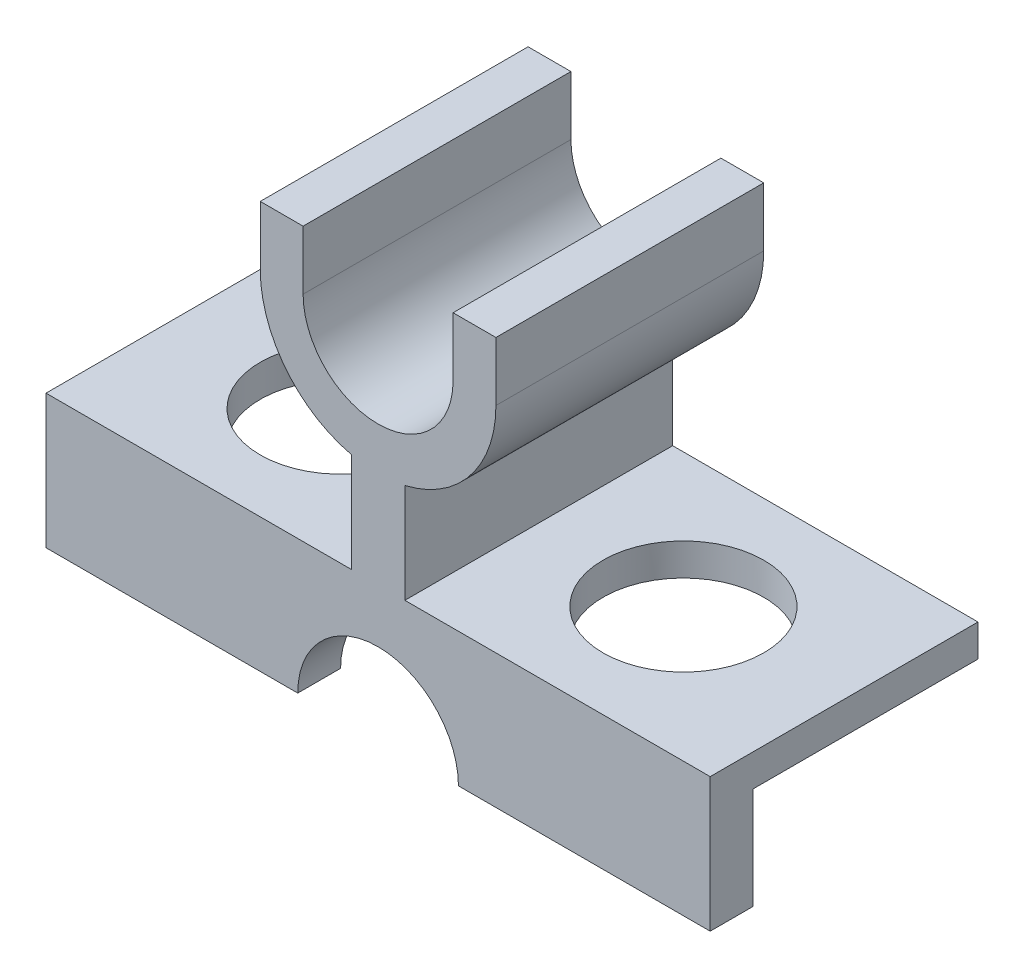
ISO-10303-21;
HEADER;
FILE_DESCRIPTION(('STEP AP214'),'2;1');
FILE_NAME('part.step','',(''),(''),'','','');
FILE_SCHEMA(('AUTOMOTIVE_DESIGN { 1 0 10303 214 1 1 1 1 }'));
ENDSEC;
DATA;
#1=APPLICATION_CONTEXT('core data for automotive mechanical design processes');
#2=APPLICATION_PROTOCOL_DEFINITION('international standard','automotive_design',2000,#1);
#3=PRODUCT_CONTEXT('',#1,'mechanical');
#4=PRODUCT('Part','Part','',(#3));
#5=PRODUCT_RELATED_PRODUCT_CATEGORY('part','',(#4));
#6=PRODUCT_DEFINITION_FORMATION('','',#4);
#7=PRODUCT_DEFINITION_CONTEXT('part definition',#1,'design');
#8=PRODUCT_DEFINITION('design','',#6,#7);
#9=PRODUCT_DEFINITION_SHAPE('','',#8);
#10=(LENGTH_UNIT() NAMED_UNIT(*) SI_UNIT(.MILLI.,.METRE.));
#11=(NAMED_UNIT(*) PLANE_ANGLE_UNIT() SI_UNIT($,.RADIAN.));
#12=(NAMED_UNIT(*) SI_UNIT($,.STERADIAN.) SOLID_ANGLE_UNIT());
#13=UNCERTAINTY_MEASURE_WITH_UNIT(LENGTH_MEASURE(1.E-05),#10,'distance_accuracy_value','');
#14=(GEOMETRIC_REPRESENTATION_CONTEXT(3) GLOBAL_UNCERTAINTY_ASSIGNED_CONTEXT((#13)) GLOBAL_UNIT_ASSIGNED_CONTEXT((#10,
#11,#12)) REPRESENTATION_CONTEXT('',''));
#15=CARTESIAN_POINT('',(0.,0.,0.));
#16=DIRECTION('',(0.,0.,1.));
#17=DIRECTION('',(1.,0.,0.));
#18=AXIS2_PLACEMENT_3D('',#15,#16,#17);
#19=CARTESIAN_POINT('',(-62.,0.,25.));
#20=DIRECTION('',(1.,0.,0.));
#21=DIRECTION('',(0.,0.,-1.));
#22=AXIS2_PLACEMENT_3D('',#19,#20,#21);
#23=PLANE('',#22);
#24=DIRECTION('',(0.,0.,1.));
#25=VECTOR('',#24,1.);
#26=CARTESIAN_POINT('',(-62.,19.,-25.));
#27=LINE('',#26,#25);
#28=CARTESIAN_POINT('',(-62.,19.,-25.));
#29=VERTEX_POINT('',#28);
#30=CARTESIAN_POINT('',(-62.,19.,17.));
#31=VERTEX_POINT('',#30);
#32=EDGE_CURVE('E54',#29,#31,#27,.T.);
#33=ORIENTED_EDGE('',*,*,#32,.T.);
#34=DIRECTION('',(0.,-1.,0.));
#35=VECTOR('',#34,1.);
#36=CARTESIAN_POINT('',(-62.,0.,17.));
#37=LINE('',#36,#35);
#38=CARTESIAN_POINT('',(-62.,0.,17.));
#39=VERTEX_POINT('',#38);
#40=EDGE_CURVE('E284',#31,#39,#37,.T.);
#41=ORIENTED_EDGE('',*,*,#40,.T.);
#42=DIRECTION('',(0.,0.,-1.));
#43=VECTOR('',#42,1.);
#44=CARTESIAN_POINT('',(-62.,0.,25.));
#45=LINE('',#44,#43);
#46=CARTESIAN_POINT('',(-62.,0.,25.));
#47=VERTEX_POINT('',#46);
#48=EDGE_CURVE('E50',#47,#39,#45,.T.);
#49=ORIENTED_EDGE('',*,*,#48,.F.);
#50=DIRECTION('',(0.,-1.,0.));
#51=VECTOR('',#50,1.);
#52=CARTESIAN_POINT('',(-62.,0.,25.));
#53=LINE('',#52,#51);
#54=CARTESIAN_POINT('',(-62.,25.,25.));
#55=VERTEX_POINT('',#54);
#56=EDGE_CURVE('E230',#55,#47,#53,.T.);
#57=ORIENTED_EDGE('',*,*,#56,.F.);
#58=DIRECTION('',(0.,0.,-1.));
#59=VECTOR('',#58,1.);
#60=CARTESIAN_POINT('',(-62.,25.,25.));
#61=LINE('',#60,#59);
#62=CARTESIAN_POINT('',(-62.,25.,-25.));
#63=VERTEX_POINT('',#62);
#64=EDGE_CURVE('E195',#55,#63,#61,.T.);
#65=ORIENTED_EDGE('',*,*,#64,.T.);
#66=DIRECTION('',(0.,-1.,0.));
#67=VECTOR('',#66,1.);
#68=CARTESIAN_POINT('',(-62.,0.,-25.));
#69=LINE('',#68,#67);
#70=EDGE_CURVE('E197',#63,#29,#69,.T.);
#71=ORIENTED_EDGE('',*,*,#70,.T.);
#72=EDGE_LOOP('',(#33,#41,#49,#57,#65,#71));
#73=FACE_BOUND('',#72,.T.);
#74=ADVANCED_FACE('F39',(#73),#23,.F.);
#75=CARTESIAN_POINT('',(-62.,0.,25.));
#76=DIRECTION('',(0.,1.,0.));
#77=DIRECTION('',(0.,0.,1.));
#78=AXIS2_PLACEMENT_3D('',#75,#76,#77);
#79=PLANE('',#78);
#80=ORIENTED_EDGE('',*,*,#48,.T.);
#81=DIRECTION('',(1.,0.,0.));
#82=VECTOR('',#81,1.);
#83=CARTESIAN_POINT('',(-62.,0.,17.));
#84=LINE('',#83,#82);
#85=CARTESIAN_POINT('',(-15.,0.,17.));
#86=VERTEX_POINT('',#85);
#87=EDGE_CURVE('E286',#39,#86,#84,.T.);
#88=ORIENTED_EDGE('',*,*,#87,.T.);
#89=DIRECTION('',(0.,0.,-1.));
#90=VECTOR('',#89,1.);
#91=CARTESIAN_POINT('',(-15.,0.,25.));
#92=LINE('',#91,#90);
#93=CARTESIAN_POINT('',(-15.,0.,25.));
#94=VERTEX_POINT('',#93);
#95=EDGE_CURVE('E270',#94,#86,#92,.T.);
#96=ORIENTED_EDGE('',*,*,#95,.F.);
#97=DIRECTION('',(1.,0.,0.));
#98=VECTOR('',#97,1.);
#99=CARTESIAN_POINT('',(-62.,0.,25.));
#100=LINE('',#99,#98);
#101=EDGE_CURVE('E121',#47,#94,#100,.T.);
#102=ORIENTED_EDGE('',*,*,#101,.F.);
#103=EDGE_LOOP('',(#80,#88,#96,#102));
#104=FACE_BOUND('',#103,.T.);
#105=ADVANCED_FACE('F350',(#104),#79,.F.);
#106=CARTESIAN_POINT('',(0.,0.,25.));
#107=DIRECTION('',(0.,0.,-1.));
#108=DIRECTION('',(-1.,0.,0.));
#109=AXIS2_PLACEMENT_3D('',#106,#107,#108);
#110=CYLINDRICAL_SURFACE('',#109,15.);
#111=ORIENTED_EDGE('',*,*,#95,.T.);
#112=CARTESIAN_POINT('',(0.,0.,17.));
#113=DIRECTION('',(0.,0.,1.));
#114=DIRECTION('',(1.,0.,0.));
#115=AXIS2_PLACEMENT_3D('',#112,#113,#114);
#116=CIRCLE('',#115,15.);
#117=CARTESIAN_POINT('',(15.,0.,17.));
#118=VERTEX_POINT('',#117);
#119=EDGE_CURVE('E203',#86,#118,#116,.F.);
#120=ORIENTED_EDGE('',*,*,#119,.T.);
#121=DIRECTION('',(0.,0.,-1.));
#122=VECTOR('',#121,1.);
#123=CARTESIAN_POINT('',(15.,0.,25.));
#124=LINE('',#123,#122);
#125=CARTESIAN_POINT('',(15.,0.,25.));
#126=VERTEX_POINT('',#125);
#127=EDGE_CURVE('E262',#126,#118,#124,.T.);
#128=ORIENTED_EDGE('',*,*,#127,.F.);
#129=CARTESIAN_POINT('',(0.,0.,25.));
#130=DIRECTION('',(0.,0.,-1.));
#131=DIRECTION('',(-1.,0.,0.));
#132=AXIS2_PLACEMENT_3D('',#129,#130,#131);
#133=CIRCLE('',#132,15.);
#134=EDGE_CURVE('E301',#94,#126,#133,.T.);
#135=ORIENTED_EDGE('',*,*,#134,.F.);
#136=EDGE_LOOP('',(#111,#120,#128,#135));
#137=FACE_BOUND('',#136,.T.);
#138=ADVANCED_FACE('F351',(#137),#110,.F.);
#139=CARTESIAN_POINT('',(15.,0.,25.));
#140=DIRECTION('',(0.,1.,0.));
#141=DIRECTION('',(0.,0.,1.));
#142=AXIS2_PLACEMENT_3D('',#139,#140,#141);
#143=PLANE('',#142);
#144=ORIENTED_EDGE('',*,*,#127,.T.);
#145=CARTESIAN_POINT('',(62.,0.,17.));
#146=VERTEX_POINT('',#145);
#147=EDGE_CURVE('E291',#118,#146,#84,.T.);
#148=ORIENTED_EDGE('',*,*,#147,.T.);
#149=DIRECTION('',(0.,0.,-1.));
#150=VECTOR('',#149,1.);
#151=CARTESIAN_POINT('',(62.,0.,25.));
#152=LINE('',#151,#150);
#153=CARTESIAN_POINT('',(62.,0.,25.));
#154=VERTEX_POINT('',#153);
#155=EDGE_CURVE('E261',#154,#146,#152,.T.);
#156=ORIENTED_EDGE('',*,*,#155,.F.);
#157=DIRECTION('',(1.,0.,0.));
#158=VECTOR('',#157,1.);
#159=CARTESIAN_POINT('',(15.,0.,25.));
#160=LINE('',#159,#158);
#161=EDGE_CURVE('E308',#126,#154,#160,.T.);
#162=ORIENTED_EDGE('',*,*,#161,.F.);
#163=EDGE_LOOP('',(#144,#148,#156,#162));
#164=FACE_BOUND('',#163,.T.);
#165=ADVANCED_FACE('F360',(#164),#143,.F.);
#166=CARTESIAN_POINT('',(62.,0.,25.));
#167=DIRECTION('',(-1.,0.,0.));
#168=DIRECTION('',(0.,0.,1.));
#169=AXIS2_PLACEMENT_3D('',#166,#167,#168);
#170=PLANE('',#169);
#171=ORIENTED_EDGE('',*,*,#155,.T.);
#172=DIRECTION('',(0.,1.,0.));
#173=VECTOR('',#172,1.);
#174=CARTESIAN_POINT('',(62.,0.,17.));
#175=LINE('',#174,#173);
#176=CARTESIAN_POINT('',(62.,19.,17.));
#177=VERTEX_POINT('',#176);
#178=EDGE_CURVE('E11',#146,#177,#175,.T.);
#179=ORIENTED_EDGE('',*,*,#178,.T.);
#180=DIRECTION('',(0.,0.,-1.));
#181=VECTOR('',#180,1.);
#182=CARTESIAN_POINT('',(62.,19.,25.));
#183=LINE('',#182,#181);
#184=CARTESIAN_POINT('',(62.,19.,-25.));
#185=VERTEX_POINT('',#184);
#186=EDGE_CURVE('E295',#177,#185,#183,.T.);
#187=ORIENTED_EDGE('',*,*,#186,.T.);
#188=DIRECTION('',(0.,1.,0.));
#189=VECTOR('',#188,1.);
#190=CARTESIAN_POINT('',(62.,0.,-25.));
#191=LINE('',#190,#189);
#192=CARTESIAN_POINT('',(62.,25.,-25.));
#193=VERTEX_POINT('',#192);
#194=EDGE_CURVE('E199',#185,#193,#191,.T.);
#195=ORIENTED_EDGE('',*,*,#194,.T.);
#196=DIRECTION('',(0.,0.,-1.));
#197=VECTOR('',#196,1.);
#198=CARTESIAN_POINT('',(62.,25.,25.));
#199=LINE('',#198,#197);
#200=CARTESIAN_POINT('',(62.,25.,25.));
#201=VERTEX_POINT('',#200);
#202=EDGE_CURVE('E256',#201,#193,#199,.T.);
#203=ORIENTED_EDGE('',*,*,#202,.F.);
#204=DIRECTION('',(0.,1.,0.));
#205=VECTOR('',#204,1.);
#206=CARTESIAN_POINT('',(62.,0.,25.));
#207=LINE('',#206,#205);
#208=EDGE_CURVE('E306',#154,#201,#207,.T.);
#209=ORIENTED_EDGE('',*,*,#208,.F.);
#210=EDGE_LOOP('',(#171,#179,#187,#195,#203,#209));
#211=FACE_BOUND('',#210,.T.);
#212=ADVANCED_FACE('F365',(#211),#170,.F.);
#213=CARTESIAN_POINT('',(5.,25.,25.));
#214=DIRECTION('',(0.,-1.,0.));
#215=DIRECTION('',(0.,0.,-1.));
#216=AXIS2_PLACEMENT_3D('',#213,#214,#215);
#217=PLANE('',#216);
#218=CARTESIAN_POINT('',(32.,25.,0.));
#219=DIRECTION('',(0.,1.,0.));
#220=DIRECTION('',(0.,0.,-1.));
#221=AXIS2_PLACEMENT_3D('',#218,#219,#220);
#222=CIRCLE('',#221,15.);
#223=CARTESIAN_POINT('',(32.,25.,-15.));
#224=VERTEX_POINT('',#223);
#225=EDGE_CURVE('E280',#224,#224,#222,.T.);
#226=ORIENTED_EDGE('',*,*,#225,.F.);
#227=EDGE_LOOP('',(#226));
#228=FACE_BOUND('',#227,.T.);
#229=DIRECTION('',(-1.,0.,0.));
#230=VECTOR('',#229,1.);
#231=CARTESIAN_POINT('',(5.,25.,-25.));
#232=LINE('',#231,#230);
#233=CARTESIAN_POINT('',(5.,25.,-25.));
#234=VERTEX_POINT('',#233);
#235=EDGE_CURVE('E201',#193,#234,#232,.T.);
#236=ORIENTED_EDGE('',*,*,#235,.T.);
#237=DIRECTION('',(0.,0.,-1.));
#238=VECTOR('',#237,1.);
#239=CARTESIAN_POINT('',(5.,25.,25.));
#240=LINE('',#239,#238);
#241=CARTESIAN_POINT('',(5.,25.,25.));
#242=VERTEX_POINT('',#241);
#243=EDGE_CURVE('E254',#242,#234,#240,.T.);
#244=ORIENTED_EDGE('',*,*,#243,.F.);
#245=DIRECTION('',(-1.,0.,0.));
#246=VECTOR('',#245,1.);
#247=CARTESIAN_POINT('',(5.,25.,25.));
#248=LINE('',#247,#246);
#249=EDGE_CURVE('E309',#201,#242,#248,.T.);
#250=ORIENTED_EDGE('',*,*,#249,.F.);
#251=ORIENTED_EDGE('',*,*,#202,.T.);
#252=EDGE_LOOP('',(#236,#244,#250,#251));
#253=FACE_BOUND('',#252,.T.);
#254=ADVANCED_FACE('F370',(#228,#253),#217,.F.);
#255=CARTESIAN_POINT('',(5.,43.5757147143715,25.));
#256=DIRECTION('',(-1.,0.,0.));
#257=DIRECTION('',(0.,-1.,0.));
#258=AXIS2_PLACEMENT_3D('',#255,#256,#257);
#259=PLANE('',#258);
#260=DIRECTION('',(0.,1.,0.));
#261=VECTOR('',#260,1.);
#262=CARTESIAN_POINT('',(5.,43.5757147143715,-25.));
#263=LINE('',#262,#261);
#264=CARTESIAN_POINT('',(5.,43.5757147143715,-25.));
#265=VERTEX_POINT('',#264);
#266=EDGE_CURVE('E202',#234,#265,#263,.T.);
#267=ORIENTED_EDGE('',*,*,#266,.T.);
#268=DIRECTION('',(0.,0.,-1.));
#269=VECTOR('',#268,1.);
#270=CARTESIAN_POINT('',(5.,43.5757147143715,25.));
#271=LINE('',#270,#269);
#272=CARTESIAN_POINT('',(5.,43.5757147143715,25.));
#273=VERTEX_POINT('',#272);
#274=EDGE_CURVE('E252',#273,#265,#271,.T.);
#275=ORIENTED_EDGE('',*,*,#274,.F.);
#276=DIRECTION('',(0.,1.,0.));
#277=VECTOR('',#276,1.);
#278=CARTESIAN_POINT('',(5.,43.5757147143715,25.));
#279=LINE('',#278,#277);
#280=EDGE_CURVE('E315',#242,#273,#279,.T.);
#281=ORIENTED_EDGE('',*,*,#280,.F.);
#282=ORIENTED_EDGE('',*,*,#243,.T.);
#283=EDGE_LOOP('',(#267,#275,#281,#282));
#284=FACE_BOUND('',#283,.T.);
#285=ADVANCED_FACE('F375',(#284),#259,.F.);
#286=CARTESIAN_POINT('',(0.,65.,25.));
#287=DIRECTION('',(0.,0.,-1.));
#288=DIRECTION('',(-1.,0.,0.));
#289=AXIS2_PLACEMENT_3D('',#286,#287,#288);
#290=CYLINDRICAL_SURFACE('',#289,22.);
#291=CARTESIAN_POINT('',(0.,65.,-25.));
#292=DIRECTION('',(0.,0.,1.));
#293=DIRECTION('',(1.,0.,0.));
#294=AXIS2_PLACEMENT_3D('',#291,#292,#293);
#295=CIRCLE('',#294,22.);
#296=CARTESIAN_POINT('',(22.,65.,-25.));
#297=VERTEX_POINT('',#296);
#298=EDGE_CURVE('E210',#265,#297,#295,.T.);
#299=ORIENTED_EDGE('',*,*,#298,.T.);
#300=DIRECTION('',(0.,0.,-1.));
#301=VECTOR('',#300,1.);
#302=CARTESIAN_POINT('',(22.,65.,25.));
#303=LINE('',#302,#301);
#304=CARTESIAN_POINT('',(22.,65.,25.));
#305=VERTEX_POINT('',#304);
#306=EDGE_CURVE('E246',#305,#297,#303,.T.);
#307=ORIENTED_EDGE('',*,*,#306,.F.);
#308=CARTESIAN_POINT('',(0.,65.,25.));
#309=DIRECTION('',(0.,0.,1.));
#310=DIRECTION('',(1.,0.,0.));
#311=AXIS2_PLACEMENT_3D('',#308,#309,#310);
#312=CIRCLE('',#311,22.);
#313=EDGE_CURVE('E314',#273,#305,#312,.T.);
#314=ORIENTED_EDGE('',*,*,#313,.F.);
#315=ORIENTED_EDGE('',*,*,#274,.T.);
#316=EDGE_LOOP('',(#299,#307,#314,#315));
#317=FACE_BOUND('',#316,.T.);
#318=ADVANCED_FACE('F378',(#317),#290,.T.);
#319=CARTESIAN_POINT('',(22.,65.,25.));
#320=DIRECTION('',(-1.,0.,0.));
#321=DIRECTION('',(0.,-1.,0.));
#322=AXIS2_PLACEMENT_3D('',#319,#320,#321);
#323=PLANE('',#322);
#324=DIRECTION('',(0.,1.,0.));
#325=VECTOR('',#324,1.);
#326=CARTESIAN_POINT('',(22.,65.,-25.));
#327=LINE('',#326,#325);
#328=CARTESIAN_POINT('',(22.,76.,-25.));
#329=VERTEX_POINT('',#328);
#330=EDGE_CURVE('E207',#297,#329,#327,.T.);
#331=ORIENTED_EDGE('',*,*,#330,.T.);
#332=DIRECTION('',(0.,0.,-1.));
#333=VECTOR('',#332,1.);
#334=CARTESIAN_POINT('',(22.,76.,25.));
#335=LINE('',#334,#333);
#336=CARTESIAN_POINT('',(22.,76.,25.));
#337=VERTEX_POINT('',#336);
#338=EDGE_CURVE('E247',#337,#329,#335,.T.);
#339=ORIENTED_EDGE('',*,*,#338,.F.);
#340=DIRECTION('',(0.,1.,0.));
#341=VECTOR('',#340,1.);
#342=CARTESIAN_POINT('',(22.,65.,25.));
#343=LINE('',#342,#341);
#344=EDGE_CURVE('E316',#305,#337,#343,.T.);
#345=ORIENTED_EDGE('',*,*,#344,.F.);
#346=ORIENTED_EDGE('',*,*,#306,.T.);
#347=EDGE_LOOP('',(#331,#339,#345,#346));
#348=FACE_BOUND('',#347,.T.);
#349=ADVANCED_FACE('F385',(#348),#323,.F.);
#350=CARTESIAN_POINT('',(14.,76.,25.));
#351=DIRECTION('',(0.,-1.,0.));
#352=DIRECTION('',(0.,0.,-1.));
#353=AXIS2_PLACEMENT_3D('',#350,#351,#352);
#354=PLANE('',#353);
#355=DIRECTION('',(-1.,0.,0.));
#356=VECTOR('',#355,1.);
#357=CARTESIAN_POINT('',(14.,76.,-25.));
#358=LINE('',#357,#356);
#359=CARTESIAN_POINT('',(14.,76.,-25.));
#360=VERTEX_POINT('',#359);
#361=EDGE_CURVE('E211',#329,#360,#358,.T.);
#362=ORIENTED_EDGE('',*,*,#361,.T.);
#363=DIRECTION('',(0.,0.,-1.));
#364=VECTOR('',#363,1.);
#365=CARTESIAN_POINT('',(14.,76.,25.));
#366=LINE('',#365,#364);
#367=CARTESIAN_POINT('',(14.,76.,25.));
#368=VERTEX_POINT('',#367);
#369=EDGE_CURVE('E242',#368,#360,#366,.T.);
#370=ORIENTED_EDGE('',*,*,#369,.F.);
#371=DIRECTION('',(-1.,0.,0.));
#372=VECTOR('',#371,1.);
#373=CARTESIAN_POINT('',(14.,76.,25.));
#374=LINE('',#373,#372);
#375=EDGE_CURVE('E318',#337,#368,#374,.T.);
#376=ORIENTED_EDGE('',*,*,#375,.F.);
#377=ORIENTED_EDGE('',*,*,#338,.T.);
#378=EDGE_LOOP('',(#362,#370,#376,#377));
#379=FACE_BOUND('',#378,.T.);
#380=ADVANCED_FACE('F390',(#379),#354,.F.);
#381=CARTESIAN_POINT('',(14.,65.,25.));
#382=DIRECTION('',(1.,0.,0.));
#383=DIRECTION('',(0.,1.,0.));
#384=AXIS2_PLACEMENT_3D('',#381,#382,#383);
#385=PLANE('',#384);
#386=DIRECTION('',(0.,-1.,0.));
#387=VECTOR('',#386,1.);
#388=CARTESIAN_POINT('',(14.,65.,-25.));
#389=LINE('',#388,#387);
#390=CARTESIAN_POINT('',(14.,65.,-25.));
#391=VERTEX_POINT('',#390);
#392=EDGE_CURVE('E213',#360,#391,#389,.T.);
#393=ORIENTED_EDGE('',*,*,#392,.T.);
#394=DIRECTION('',(0.,0.,-1.));
#395=VECTOR('',#394,1.);
#396=CARTESIAN_POINT('',(14.,65.,25.));
#397=LINE('',#396,#395);
#398=CARTESIAN_POINT('',(14.,65.,25.));
#399=VERTEX_POINT('',#398);
#400=EDGE_CURVE('E238',#399,#391,#397,.T.);
#401=ORIENTED_EDGE('',*,*,#400,.F.);
#402=DIRECTION('',(0.,-1.,0.));
#403=VECTOR('',#402,1.);
#404=CARTESIAN_POINT('',(14.,65.,25.));
#405=LINE('',#404,#403);
#406=EDGE_CURVE('E319',#368,#399,#405,.T.);
#407=ORIENTED_EDGE('',*,*,#406,.F.);
#408=ORIENTED_EDGE('',*,*,#369,.T.);
#409=EDGE_LOOP('',(#393,#401,#407,#408));
#410=FACE_BOUND('',#409,.T.);
#411=ADVANCED_FACE('F392',(#410),#385,.F.);
#412=CARTESIAN_POINT('',(0.,65.,25.));
#413=DIRECTION('',(0.,0.,-1.));
#414=DIRECTION('',(-1.,0.,0.));
#415=AXIS2_PLACEMENT_3D('',#412,#413,#414);
#416=CYLINDRICAL_SURFACE('',#415,14.);
#417=CARTESIAN_POINT('',(0.,65.,-25.));
#418=DIRECTION('',(0.,0.,-1.));
#419=DIRECTION('',(1.,0.,0.));
#420=AXIS2_PLACEMENT_3D('',#417,#418,#419);
#421=CIRCLE('',#420,14.);
#422=CARTESIAN_POINT('',(-14.,65.,-25.));
#423=VERTEX_POINT('',#422);
#424=EDGE_CURVE('E214',#391,#423,#421,.T.);
#425=ORIENTED_EDGE('',*,*,#424,.T.);
#426=DIRECTION('',(0.,0.,-1.));
#427=VECTOR('',#426,1.);
#428=CARTESIAN_POINT('',(-14.,65.,25.));
#429=LINE('',#428,#427);
#430=CARTESIAN_POINT('',(-14.,65.,25.));
#431=VERTEX_POINT('',#430);
#432=EDGE_CURVE('E240',#431,#423,#429,.T.);
#433=ORIENTED_EDGE('',*,*,#432,.F.);
#434=CARTESIAN_POINT('',(0.,65.,25.));
#435=DIRECTION('',(0.,0.,-1.));
#436=DIRECTION('',(1.,0.,0.));
#437=AXIS2_PLACEMENT_3D('',#434,#435,#436);
#438=CIRCLE('',#437,14.);
#439=EDGE_CURVE('E325',#399,#431,#438,.T.);
#440=ORIENTED_EDGE('',*,*,#439,.F.);
#441=ORIENTED_EDGE('',*,*,#400,.T.);
#442=EDGE_LOOP('',(#425,#433,#440,#441));
#443=FACE_BOUND('',#442,.T.);
#444=ADVANCED_FACE('F399',(#443),#416,.F.);
#445=CARTESIAN_POINT('',(-14.,65.,25.));
#446=DIRECTION('',(-1.,0.,0.));
#447=DIRECTION('',(0.,0.,1.));
#448=AXIS2_PLACEMENT_3D('',#445,#446,#447);
#449=PLANE('',#448);
#450=DIRECTION('',(0.,1.,0.));
#451=VECTOR('',#450,1.);
#452=CARTESIAN_POINT('',(-14.,65.,-25.));
#453=LINE('',#452,#451);
#454=CARTESIAN_POINT('',(-14.,76.,-25.));
#455=VERTEX_POINT('',#454);
#456=EDGE_CURVE('E220',#423,#455,#453,.T.);
#457=ORIENTED_EDGE('',*,*,#456,.T.);
#458=DIRECTION('',(0.,0.,-1.));
#459=VECTOR('',#458,1.);
#460=CARTESIAN_POINT('',(-14.,76.,25.));
#461=LINE('',#460,#459);
#462=CARTESIAN_POINT('',(-14.,76.,25.));
#463=VERTEX_POINT('',#462);
#464=EDGE_CURVE('E231',#463,#455,#461,.T.);
#465=ORIENTED_EDGE('',*,*,#464,.F.);
#466=DIRECTION('',(0.,1.,0.));
#467=VECTOR('',#466,1.);
#468=CARTESIAN_POINT('',(-14.,65.,25.));
#469=LINE('',#468,#467);
#470=EDGE_CURVE('E322',#431,#463,#469,.T.);
#471=ORIENTED_EDGE('',*,*,#470,.F.);
#472=ORIENTED_EDGE('',*,*,#432,.T.);
#473=EDGE_LOOP('',(#457,#465,#471,#472));
#474=FACE_BOUND('',#473,.T.);
#475=ADVANCED_FACE('F398',(#474),#449,.F.);
#476=CARTESIAN_POINT('',(-14.,76.,25.));
#477=DIRECTION('',(0.,-1.,0.));
#478=DIRECTION('',(0.,0.,-1.));
#479=AXIS2_PLACEMENT_3D('',#476,#477,#478);
#480=PLANE('',#479);
#481=DIRECTION('',(-1.,0.,0.));
#482=VECTOR('',#481,1.);
#483=CARTESIAN_POINT('',(-14.,76.,-25.));
#484=LINE('',#483,#482);
#485=CARTESIAN_POINT('',(-22.,76.,-25.));
#486=VERTEX_POINT('',#485);
#487=EDGE_CURVE('E218',#455,#486,#484,.T.);
#488=ORIENTED_EDGE('',*,*,#487,.T.);
#489=DIRECTION('',(0.,0.,-1.));
#490=VECTOR('',#489,1.);
#491=CARTESIAN_POINT('',(-22.,76.,25.));
#492=LINE('',#491,#490);
#493=CARTESIAN_POINT('',(-22.,76.,25.));
#494=VERTEX_POINT('',#493);
#495=EDGE_CURVE('E232',#494,#486,#492,.T.);
#496=ORIENTED_EDGE('',*,*,#495,.F.);
#497=DIRECTION('',(-1.,0.,0.));
#498=VECTOR('',#497,1.);
#499=CARTESIAN_POINT('',(-14.,76.,25.));
#500=LINE('',#499,#498);
#501=EDGE_CURVE('E326',#463,#494,#500,.T.);
#502=ORIENTED_EDGE('',*,*,#501,.F.);
#503=ORIENTED_EDGE('',*,*,#464,.T.);
#504=EDGE_LOOP('',(#488,#496,#502,#503));
#505=FACE_BOUND('',#504,.T.);
#506=ADVANCED_FACE('F335',(#505),#480,.F.);
#507=CARTESIAN_POINT('',(-22.,65.,25.));
#508=DIRECTION('',(1.,0.,0.));
#509=DIRECTION('',(0.,0.,-1.));
#510=AXIS2_PLACEMENT_3D('',#507,#508,#509);
#511=PLANE('',#510);
#512=DIRECTION('',(0.,-1.,0.));
#513=VECTOR('',#512,1.);
#514=CARTESIAN_POINT('',(-22.,65.,-25.));
#515=LINE('',#514,#513);
#516=CARTESIAN_POINT('',(-22.,65.,-25.));
#517=VERTEX_POINT('',#516);
#518=EDGE_CURVE('E222',#486,#517,#515,.T.);
#519=ORIENTED_EDGE('',*,*,#518,.T.);
#520=DIRECTION('',(0.,0.,-1.));
#521=VECTOR('',#520,1.);
#522=CARTESIAN_POINT('',(-22.,65.,25.));
#523=LINE('',#522,#521);
#524=CARTESIAN_POINT('',(-22.,65.,25.));
#525=VERTEX_POINT('',#524);
#526=EDGE_CURVE('E187',#525,#517,#523,.T.);
#527=ORIENTED_EDGE('',*,*,#526,.F.);
#528=DIRECTION('',(0.,-1.,0.));
#529=VECTOR('',#528,1.);
#530=CARTESIAN_POINT('',(-22.,65.,25.));
#531=LINE('',#530,#529);
#532=EDGE_CURVE('E177',#494,#525,#531,.T.);
#533=ORIENTED_EDGE('',*,*,#532,.F.);
#534=ORIENTED_EDGE('',*,*,#495,.T.);
#535=EDGE_LOOP('',(#519,#527,#533,#534));
#536=FACE_BOUND('',#535,.T.);
#537=ADVANCED_FACE('F336',(#536),#511,.F.);
#538=CARTESIAN_POINT('',(0.,65.,25.));
#539=DIRECTION('',(0.,0.,-1.));
#540=DIRECTION('',(-1.,0.,0.));
#541=AXIS2_PLACEMENT_3D('',#538,#539,#540);
#542=CYLINDRICAL_SURFACE('',#541,22.);
#543=CARTESIAN_POINT('',(0.,65.,-25.));
#544=DIRECTION('',(0.,0.,1.));
#545=DIRECTION('',(1.,0.,0.));
#546=AXIS2_PLACEMENT_3D('',#543,#544,#545);
#547=CIRCLE('',#546,22.);
#548=CARTESIAN_POINT('',(-5.00000000000001,43.5757147143715,-25.));
#549=VERTEX_POINT('',#548);
#550=EDGE_CURVE('E183',#517,#549,#547,.T.);
#551=ORIENTED_EDGE('',*,*,#550,.T.);
#552=DIRECTION('',(0.,0.,-1.));
#553=VECTOR('',#552,1.);
#554=CARTESIAN_POINT('',(-5.00000000000001,43.5757147143715,25.));
#555=LINE('',#554,#553);
#556=CARTESIAN_POINT('',(-5.00000000000001,43.5757147143715,25.));
#557=VERTEX_POINT('',#556);
#558=EDGE_CURVE('E185',#557,#549,#555,.T.);
#559=ORIENTED_EDGE('',*,*,#558,.F.);
#560=CARTESIAN_POINT('',(0.,65.,25.));
#561=DIRECTION('',(0.,0.,1.));
#562=DIRECTION('',(1.,0.,0.));
#563=AXIS2_PLACEMENT_3D('',#560,#561,#562);
#564=CIRCLE('',#563,22.);
#565=EDGE_CURVE('E166',#525,#557,#564,.T.);
#566=ORIENTED_EDGE('',*,*,#565,.F.);
#567=ORIENTED_EDGE('',*,*,#526,.T.);
#568=EDGE_LOOP('',(#551,#559,#566,#567));
#569=FACE_BOUND('',#568,.T.);
#570=ADVANCED_FACE('F181',(#569),#542,.T.);
#571=CARTESIAN_POINT('',(-5.,43.5757147143715,25.));
#572=DIRECTION('',(1.,0.,0.));
#573=DIRECTION('',(0.,1.,0.));
#574=AXIS2_PLACEMENT_3D('',#571,#572,#573);
#575=PLANE('',#574);
#576=DIRECTION('',(0.,-1.,0.));
#577=VECTOR('',#576,1.);
#578=CARTESIAN_POINT('',(-5.,43.5757147143715,-25.));
#579=LINE('',#578,#577);
#580=CARTESIAN_POINT('',(-5.,25.,-25.));
#581=VERTEX_POINT('',#580);
#582=EDGE_CURVE('E221',#549,#581,#579,.T.);
#583=ORIENTED_EDGE('',*,*,#582,.T.);
#584=DIRECTION('',(0.,0.,-1.));
#585=VECTOR('',#584,1.);
#586=CARTESIAN_POINT('',(-5.,25.,25.));
#587=LINE('',#586,#585);
#588=CARTESIAN_POINT('',(-5.,25.,25.));
#589=VERTEX_POINT('',#588);
#590=EDGE_CURVE('E188',#589,#581,#587,.T.);
#591=ORIENTED_EDGE('',*,*,#590,.F.);
#592=DIRECTION('',(0.,-1.,0.));
#593=VECTOR('',#592,1.);
#594=CARTESIAN_POINT('',(-5.,43.5757147143715,25.));
#595=LINE('',#594,#593);
#596=EDGE_CURVE('E172',#557,#589,#595,.T.);
#597=ORIENTED_EDGE('',*,*,#596,.F.);
#598=ORIENTED_EDGE('',*,*,#558,.T.);
#599=EDGE_LOOP('',(#583,#591,#597,#598));
#600=FACE_BOUND('',#599,.T.);
#601=ADVANCED_FACE('F192',(#600),#575,.F.);
#602=CARTESIAN_POINT('',(-62.,25.,25.));
#603=DIRECTION('',(0.,-1.,0.));
#604=DIRECTION('',(0.,0.,-1.));
#605=AXIS2_PLACEMENT_3D('',#602,#603,#604);
#606=PLANE('',#605);
#607=CARTESIAN_POINT('',(-32.,25.,0.));
#608=DIRECTION('',(0.,1.,0.));
#609=DIRECTION('',(0.,0.,1.));
#610=AXIS2_PLACEMENT_3D('',#607,#608,#609);
#611=CIRCLE('',#610,15.);
#612=CARTESIAN_POINT('',(-32.,25.,15.));
#613=VERTEX_POINT('',#612);
#614=EDGE_CURVE('E275',#613,#613,#611,.T.);
#615=ORIENTED_EDGE('',*,*,#614,.F.);
#616=EDGE_LOOP('',(#615));
#617=FACE_BOUND('',#616,.T.);
#618=DIRECTION('',(-1.,0.,0.));
#619=VECTOR('',#618,1.);
#620=CARTESIAN_POINT('',(-62.,25.,-25.));
#621=LINE('',#620,#619);
#622=EDGE_CURVE('E113',#581,#63,#621,.T.);
#623=ORIENTED_EDGE('',*,*,#622,.T.);
#624=ORIENTED_EDGE('',*,*,#64,.F.);
#625=DIRECTION('',(-1.,0.,0.));
#626=VECTOR('',#625,1.);
#627=CARTESIAN_POINT('',(-62.,25.,25.));
#628=LINE('',#627,#626);
#629=EDGE_CURVE('E63',#589,#55,#628,.T.);
#630=ORIENTED_EDGE('',*,*,#629,.F.);
#631=ORIENTED_EDGE('',*,*,#590,.T.);
#632=EDGE_LOOP('',(#623,#624,#630,#631));
#633=FACE_BOUND('',#632,.T.);
#634=ADVANCED_FACE('F342',(#617,#633),#606,.F.);
#635=CARTESIAN_POINT('',(0.,65.,25.));
#636=DIRECTION('',(0.,0.,1.));
#637=DIRECTION('',(1.,0.,0.));
#638=AXIS2_PLACEMENT_3D('',#635,#636,#637);
#639=PLANE('',#638);
#640=ORIENTED_EDGE('',*,*,#56,.T.);
#641=ORIENTED_EDGE('',*,*,#101,.T.);
#642=ORIENTED_EDGE('',*,*,#134,.T.);
#643=ORIENTED_EDGE('',*,*,#161,.T.);
#644=ORIENTED_EDGE('',*,*,#208,.T.);
#645=ORIENTED_EDGE('',*,*,#249,.T.);
#646=ORIENTED_EDGE('',*,*,#280,.T.);
#647=ORIENTED_EDGE('',*,*,#313,.T.);
#648=ORIENTED_EDGE('',*,*,#344,.T.);
#649=ORIENTED_EDGE('',*,*,#375,.T.);
#650=ORIENTED_EDGE('',*,*,#406,.T.);
#651=ORIENTED_EDGE('',*,*,#439,.T.);
#652=ORIENTED_EDGE('',*,*,#470,.T.);
#653=ORIENTED_EDGE('',*,*,#501,.T.);
#654=ORIENTED_EDGE('',*,*,#532,.T.);
#655=ORIENTED_EDGE('',*,*,#565,.T.);
#656=ORIENTED_EDGE('',*,*,#596,.T.);
#657=ORIENTED_EDGE('',*,*,#629,.T.);
#658=EDGE_LOOP('',(#640,#641,#642,#643,#644,#645,#646,#647,#648,#649,#650,#651,#652,#653,#654,
#655,#656,#657));
#659=FACE_BOUND('',#658,.T.);
#660=ADVANCED_FACE('F171',(#659),#639,.T.);
#661=CARTESIAN_POINT('',(0.,65.,-25.));
#662=DIRECTION('',(0.,0.,1.));
#663=DIRECTION('',(1.,0.,0.));
#664=AXIS2_PLACEMENT_3D('',#661,#662,#663);
#665=PLANE('',#664);
#666=ORIENTED_EDGE('',*,*,#194,.F.);
#667=DIRECTION('',(1.,0.,0.));
#668=VECTOR('',#667,1.);
#669=CARTESIAN_POINT('',(-62.,19.,-25.));
#670=LINE('',#669,#668);
#671=EDGE_CURVE('E290',#29,#185,#670,.T.);
#672=ORIENTED_EDGE('',*,*,#671,.F.);
#673=ORIENTED_EDGE('',*,*,#70,.F.);
#674=ORIENTED_EDGE('',*,*,#622,.F.);
#675=ORIENTED_EDGE('',*,*,#582,.F.);
#676=ORIENTED_EDGE('',*,*,#550,.F.);
#677=ORIENTED_EDGE('',*,*,#518,.F.);
#678=ORIENTED_EDGE('',*,*,#487,.F.);
#679=ORIENTED_EDGE('',*,*,#456,.F.);
#680=ORIENTED_EDGE('',*,*,#424,.F.);
#681=ORIENTED_EDGE('',*,*,#392,.F.);
#682=ORIENTED_EDGE('',*,*,#361,.F.);
#683=ORIENTED_EDGE('',*,*,#330,.F.);
#684=ORIENTED_EDGE('',*,*,#298,.F.);
#685=ORIENTED_EDGE('',*,*,#266,.F.);
#686=ORIENTED_EDGE('',*,*,#235,.F.);
#687=EDGE_LOOP('',(#666,#672,#673,#674,#675,#676,#677,#678,#679,#680,#681,#682,#683,#684,#685,#686));
#688=FACE_BOUND('',#687,.T.);
#689=ADVANCED_FACE('F338',(#688),#665,.F.);
#690=CARTESIAN_POINT('',(-62.,0.,17.));
#691=DIRECTION('',(0.,0.,1.));
#692=DIRECTION('',(1.,0.,0.));
#693=AXIS2_PLACEMENT_3D('',#690,#691,#692);
#694=PLANE('',#693);
#695=ORIENTED_EDGE('',*,*,#87,.F.);
#696=ORIENTED_EDGE('',*,*,#40,.F.);
#697=DIRECTION('',(1.,0.,0.));
#698=VECTOR('',#697,1.);
#699=CARTESIAN_POINT('',(-62.,19.,17.));
#700=LINE('',#699,#698);
#701=EDGE_CURVE('E294',#31,#177,#700,.T.);
#702=ORIENTED_EDGE('',*,*,#701,.T.);
#703=ORIENTED_EDGE('',*,*,#178,.F.);
#704=ORIENTED_EDGE('',*,*,#147,.F.);
#705=ORIENTED_EDGE('',*,*,#119,.F.);
#706=EDGE_LOOP('',(#695,#696,#702,#703,#704,#705));
#707=FACE_BOUND('',#706,.T.);
#708=ADVANCED_FACE('F414',(#707),#694,.F.);
#709=CARTESIAN_POINT('',(-62.,19.,-25.));
#710=DIRECTION('',(0.,1.,0.));
#711=DIRECTION('',(0.,0.,1.));
#712=AXIS2_PLACEMENT_3D('',#709,#710,#711);
#713=PLANE('',#712);
#714=CARTESIAN_POINT('',(-32.,19.,0.));
#715=DIRECTION('',(0.,1.,0.));
#716=DIRECTION('',(0.,0.,1.));
#717=AXIS2_PLACEMENT_3D('',#714,#715,#716);
#718=CIRCLE('',#717,15.);
#719=CARTESIAN_POINT('',(-32.,19.,15.));
#720=VERTEX_POINT('',#719);
#721=EDGE_CURVE('E45',#720,#720,#718,.T.);
#722=ORIENTED_EDGE('',*,*,#721,.T.);
#723=EDGE_LOOP('',(#722));
#724=FACE_BOUND('',#723,.T.);
#725=CARTESIAN_POINT('',(32.,19.,0.));
#726=DIRECTION('',(0.,1.,0.));
#727=DIRECTION('',(0.,0.,1.));
#728=AXIS2_PLACEMENT_3D('',#725,#726,#727);
#729=CIRCLE('',#728,15.);
#730=CARTESIAN_POINT('',(32.,19.,15.));
#731=VERTEX_POINT('',#730);
#732=EDGE_CURVE('E269',#731,#731,#729,.T.);
#733=ORIENTED_EDGE('',*,*,#732,.T.);
#734=EDGE_LOOP('',(#733));
#735=FACE_BOUND('',#734,.T.);
#736=ORIENTED_EDGE('',*,*,#701,.F.);
#737=ORIENTED_EDGE('',*,*,#32,.F.);
#738=ORIENTED_EDGE('',*,*,#671,.T.);
#739=ORIENTED_EDGE('',*,*,#186,.F.);
#740=EDGE_LOOP('',(#736,#737,#738,#739));
#741=FACE_BOUND('',#740,.T.);
#742=ADVANCED_FACE('F411',(#724,#735,#741),#713,.F.);
#743=CARTESIAN_POINT('',(32.,0.,0.));
#744=DIRECTION('',(0.,1.,0.));
#745=DIRECTION('',(0.,0.,1.));
#746=AXIS2_PLACEMENT_3D('',#743,#744,#745);
#747=CYLINDRICAL_SURFACE('',#746,15.);
#748=ORIENTED_EDGE('',*,*,#225,.T.);
#749=EDGE_LOOP('',(#748));
#750=FACE_BOUND('',#749,.T.);
#751=ORIENTED_EDGE('',*,*,#732,.F.);
#752=EDGE_LOOP('',(#751));
#753=FACE_BOUND('',#752,.T.);
#754=ADVANCED_FACE('F416',(#750,#753),#747,.F.);
#755=CARTESIAN_POINT('',(-32.,0.,0.));
#756=DIRECTION('',(0.,1.,0.));
#757=DIRECTION('',(0.,0.,1.));
#758=AXIS2_PLACEMENT_3D('',#755,#756,#757);
#759=CYLINDRICAL_SURFACE('',#758,15.);
#760=ORIENTED_EDGE('',*,*,#614,.T.);
#761=EDGE_LOOP('',(#760));
#762=FACE_BOUND('',#761,.T.);
#763=ORIENTED_EDGE('',*,*,#721,.F.);
#764=EDGE_LOOP('',(#763));
#765=FACE_BOUND('',#764,.T.);
#766=ADVANCED_FACE('F422',(#762,#765),#759,.F.);
#767=CLOSED_SHELL('',(#74,#105,#138,#165,#212,#254,#285,#318,#349,#380,#411,#444,#475,#506,#537,
#570,#601,#634,#660,#689,#708,#742,#754,#766));
#768=MANIFOLD_SOLID_BREP('B2',#767);
#769=ADVANCED_BREP_SHAPE_REPRESENTATION('',(#18,#768),#14);
#770=SHAPE_DEFINITION_REPRESENTATION(#9,#769);
ENDSEC;
END-ISO-10303-21;
